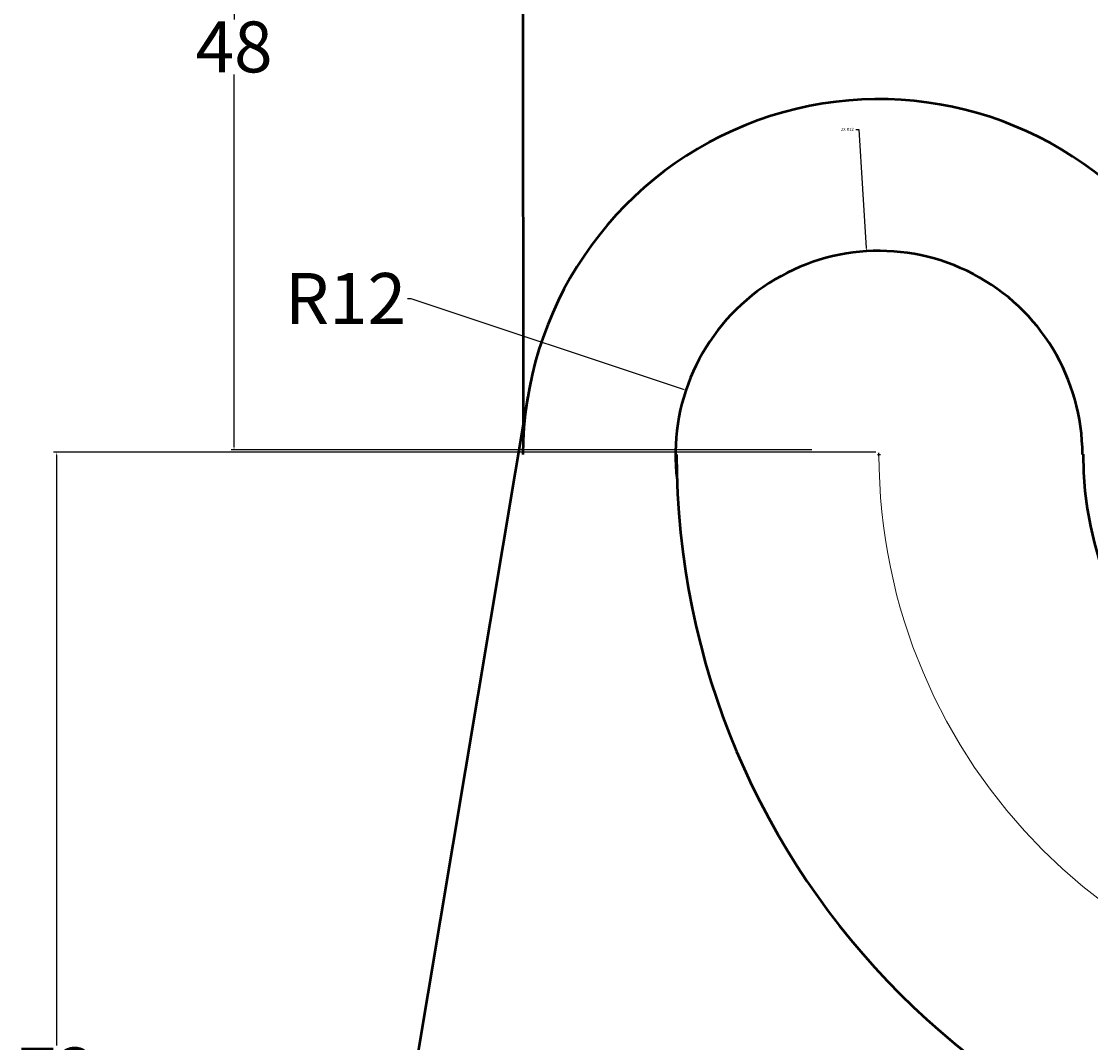
# Model space of a CAD drawing. Units: millimetres. Extents: x -50 to 109, y -46 to 152.
# Tile 10 of 18: x -50 to 13, y 32 to 92. Entities that reach past the tile are written whole.
import ezdxf

# ---------------------------------------------------------------- set-up
doc = ezdxf.new("R2010")
doc.units = ezdxf.units.MM
doc.header["$MEASUREMENT"] = 0
doc.linetypes.add('CENTER', pattern=[50.8, 31.75, -6.35, 6.35, -6.35])
for name, color, linetype, lineweight in [('M-CNTR', 1, 'CENTER', 18), ('M-DIMS', 2, 'Continuous', 25), ('M-OUTL', 7, 'Continuous', 50)]:
    doc.layers.add(name, color=color, linetype=linetype, lineweight=lineweight)
doc.styles.get("Standard").update_dxf_attribs({"font": 'arial.ttf'})
doc.dimstyles.get("Standard").update_dxf_attribs({"dimtxt": 0.18, "dimasz": 0.18, "dimexe": 0.18, "dimexo": 0.0625, "dimgap": 0.09, "dimtad": 0, "dimtih": 1, "dimtoh": 1, "dimdec": 4, "dimzin": 0, "dimdsep": 46, "dimtxsty": 'Standard', "dimcen": 0.09, "dimadec": 0, "dimazin": 0, "dimtfac": 1, "dimtdec": 4, "dimtofl": 0, "dimtmove": 0, "dimatfit": 3, "dimfxl": 1, "dimtolj": 1, "dimtzin": 0, "dimarcsym": 0})

# ---------------------------------------------------------------- blocks, each defined once
blk = doc.blocks.new('*D14')
at = {"layer": 'Defpoints', "color": 0, "transparency": 16777216}
for p in [(-11.255, 70.032), (0.13, 66.24)]:
    blk.add_point(p, dxfattribs=at)
at = {"layer": 'M-DIMS', "color": 0, "lineweight": -2, "transparency": 16777216}
for p, q in [((-27.667, 75.438), (-27.487, 75.438)), ((-27.487, 75.438), (-11.426, 70.089)), ((0.04, 66.24), (0.22, 66.24)), ((0.13, 66.15), (0.13, 66.33))]:
    blk.add_line(p, q, dxfattribs=at)
at = {"layer": 'M-DIMS', "color": 0, "transparency": 16777216}
blk.add_solid([(-11.416, 70.117), (-11.435, 70.06), (-11.255, 70.032)], dxfattribs=at)
at = {"layer": 'M-DIMS', "color": 0, "transparency": 16777216, "insert": (-31.325, 75.438), "char_height": 0.18, "attachment_point": 5}
blk.add_mtext('\\A1;{\\H16.66667x;R12}', dxfattribs=at)
blk = doc.blocks.new('*D15')
at = {"layer": 'Defpoints', "color": 0, "transparency": 16777216}
for p in [(-4.766, 114.02), (-37.902, 66.508), (-3.772, 66.508)]:
    blk.add_point(p, dxfattribs=at)
at = {"layer": 'M-DIMS', "color": 0, "lineweight": -2, "transparency": 16777216}
for p, q in [((-4.828, 114.02), (-38.082, 114.02)), ((-37.902, 113.84), (-37.902, 91.886)), ((-37.902, 66.688), (-37.902, 88.643)), ((-3.834, 66.508), (-38.082, 66.508))]:
    blk.add_line(p, q, dxfattribs=at)
at = {"layer": 'M-DIMS', "color": 0, "transparency": 16777216}
for points in [[(-37.932, 113.84), (-37.872, 113.84), (-37.902, 114.02)], [(-37.932, 66.688), (-37.872, 66.688), (-37.902, 66.508)]]:
    blk.add_solid(points, dxfattribs=at)
at = {"layer": 'M-DIMS', "color": 0, "transparency": 16777216, "insert": (-37.902, 90.264), "char_height": 0.18, "attachment_point": 5}
blk.add_mtext('\\A1;{\\H16.66667x;48}', dxfattribs=at)
blk = doc.blocks.new('*D25')
at = {"layer": 'Defpoints', "color": 0, "transparency": 16777216}
for p in [(0.007, 66.376), (-48.373, -6.811), (-0.299, -6.811)]:
    blk.add_point(p, dxfattribs=at)
at = {"layer": 'M-DIMS', "color": 0, "lineweight": -2, "transparency": 16777216}
for p, q in [((-0.056, 66.376), (-48.553, 66.376)), ((-48.373, 66.196), (-48.373, 31.405)), ((-48.373, -6.631), (-48.373, 28.16)), ((-0.361, -6.811), (-48.553, -6.811))]:
    blk.add_line(p, q, dxfattribs=at)
at = {"layer": 'M-DIMS', "color": 0, "transparency": 16777216}
for points in [[(-48.403, 66.196), (-48.343, 66.196), (-48.373, 66.376)], [(-48.403, -6.631), (-48.343, -6.631), (-48.373, -6.811)]]:
    blk.add_solid(points, dxfattribs=at)
at = {"layer": 'M-DIMS', "color": 0, "transparency": 16777216, "insert": (-48.373, 29.782), "char_height": 0.18, "attachment_point": 5}
blk.add_mtext('\\A1;{\\H16.66667x;73}', dxfattribs=at)
blk = doc.blocks.new('*D32')
at = {"layer": 'Defpoints', "color": 0, "transparency": 16777216}
for p in [(-0.611, 78.217), (0.13, 66.24)]:
    blk.add_point(p, dxfattribs=at)
at = {"layer": 'M-DIMS', "color": 0, "lineweight": -2, "transparency": 16777216}
for p, q in [((-1.236, 85.404), (-1.056, 85.404)), ((-1.056, 85.404), (-0.622, 78.397)), ((0.04, 66.24), (0.22, 66.24)), ((0.13, 66.15), (0.13, 66.33))]:
    blk.add_line(p, q, dxfattribs=at)
at = {"layer": 'M-DIMS', "color": 0, "transparency": 16777216}
blk.add_solid([(-0.592, 78.399), (-0.652, 78.395), (-0.611, 78.217)], dxfattribs=at)
at = {"layer": 'M-DIMS', "color": 0, "transparency": 16777216, "insert": (-1.735, 85.404), "char_height": 0.18, "attachment_point": 5}
blk.add_mtext('\\A1;2X R12', dxfattribs=at)

msp = doc.modelspace()

# ---------------------------------------------------------------- linework, layer by layer
at = {"layer": 'M-CNTR'}
msp.add_arc((33.1307, 66.24997), 33, 180.0142817, 359.9857183, dxfattribs=at)
at = {"layer": 'M-OUTL'}
for p, q in [((-20.89964, 114.2123), (-20.84638, 67.15852)), ((-20.5811, 69.65018), (-32.48503, -1.5038)), ((-11.86985, 66.24174), (-11.803, 66.24174)), ((12.13015, 66.24174), (12.16988, 66.24174))]:
    msp.add_line(p, q, dxfattribs=at)
for centre, radius, start, end in [((0.13105, 66.18507), 21, 44.1589895, 179.8453805), ((0.13015, 66.24022), 12, 0.0072821, 187.0790704), ((33.197, 66.24997), 45, 180.0104732, 359.9895268), ((33.16988, 66.24975), 21, 180, 0)]:
    msp.add_arc(centre, radius, start, end, dxfattribs=at)

# ---------------------------------------------------------------- dimensions: what is measured, and where the dimension line sits
at = {"layer": 'M-DIMS'}
for base, p1, p2, text, picture, middle in [((-37.90219, 66.50813), (-4.76572, 114.02048), (-3.77162, 66.50813), '{\\H16.66667x;48}', '*D15', (-37.90219, 90.26431)), ((-48.37276, -6.81116), (0.00669, 66.37611), (-0.2986, -6.81116), '{\\H16.66667x;73}', '*D25', (-48.37276, 29.78248))]:
    dim = msp.add_linear_dim(base=base, p1=p1, p2=p2, angle=90, text=text, dimstyle='Standard', override={"dimclrd": 0, "dimclre": 0, "dimclrt": 0}, dxfattribs=at)
    dim.commit()
    dim.dimension.update_dxf_attribs({"geometry": picture, "text_midpoint": middle})
for mpoint, text, override, picture, middle in [((-0.61102, 78.21731), '2X <>', {"dimdec": 0, "dimlfac": 1, "dimrnd": 0, "dimzin": 0, "dimdsep": 46, "dimlunit": 2}, '*D32', (-1.73477, 85.40356)), ((-11.25503, 70.03201), '{\\H16.66667x;R12}', {"dimclrd": 0, "dimclre": 0, "dimclrt": 0}, '*D14', (-31.32546, 75.43787))]:
    dim = msp.add_radius_dim(center=(0.13015, 66.24022), mpoint=mpoint, text=text, dimstyle='Standard', override=override, dxfattribs=at)
    dim.commit()
    dim.dimension.update_dxf_attribs({"geometry": picture, "text_midpoint": middle, "dimtype": 164})

doc.saveas('drawing.dxf')
